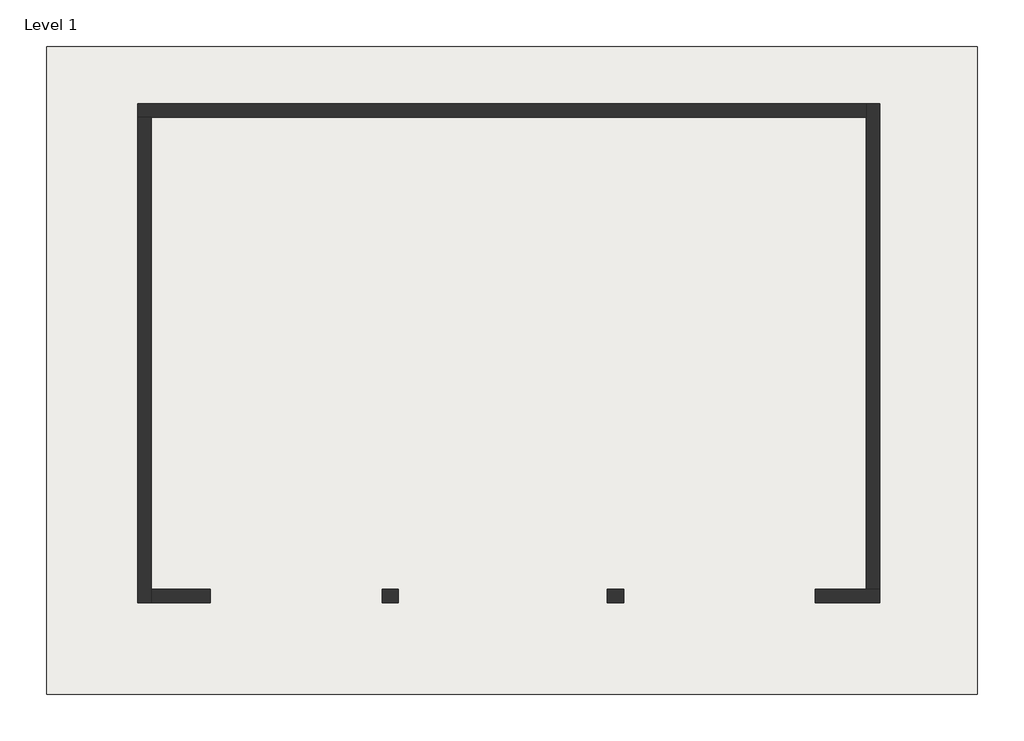
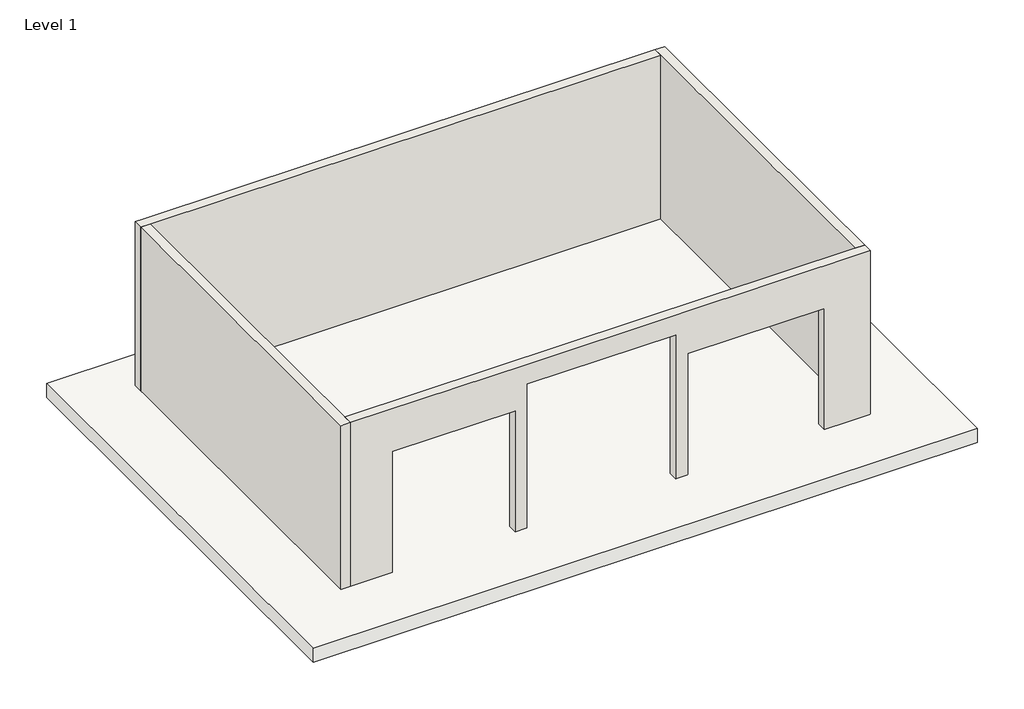
# One storey: 4 walls, 1 slab.
"""IFC4 building model written with IfcOpenShell, lengths in millimetres."""

from ifc_helpers import new_model, si_unit, frame, origin, place, context, project, spatial, polyline, outline, extrude, faceted_brep, element, save

model = new_model("IFC4")

# Units and contexts
model_context = context("Model", 3, world=origin())
ifc_project = project(units=[si_unit("LENGTHUNIT", "METRE", prefix="MILLI")], contexts=[model_context])

# Site, building, storey
site = spatial("IfcSite", under=ifc_project)
building = spatial("IfcBuilding", under=site)
storey = spatial("IfcBuildingStorey", under=building, Name="Level 1", Elevation=0.0)

# Slab
placement = place(None, origin())
element("IfcSlab", 1, ObjectType="Generic - 12\"", at=placement, inside=storey, context=model_context, shape_type="SweptSolid", body=[
    extrude(outline(polyline([(1630.1130714, 10293.742324), (1630.1130714, 540.142324), (-12390.6869286, 540.142324), (-12390.6869286, 10293.742324), (1630.1130714, 10293.742324)])), frame((0.0, 0.0, -304.8), z_axis=(0.0, 0.0, 1.0), x_axis=(1.0, 0.0, 0.0)), (0.0, 0.0, 1.0), 304.8),
])

# Walls
element("IfcWall", 2, ObjectType="Generic - 8\"", at=placement, inside=storey, context=model_context, shape_type="Brep", body=[
    faceted_brep([(-11016.1183714, 9229.4236997, 0.0), (-10812.9183714, 9229.4236997, 0.0), (-43.3183714, 9229.4236997, 0.0), (-43.3183714, 9229.4236997, 3657.6), (-10812.9183714, 9229.4236997, 3657.6), (-11016.1183714, 9229.4236997, 3657.6), (-11016.1183714, 9432.6236997, 0.0), (-11016.1183714, 9432.6236997, 3657.6), (-10812.9183714, 9432.6236997, 3657.6), (-43.3183714, 9432.6236997, 3657.6), (-43.3183714, 9432.6236997, 0.0)], [[[0, 1, 2, 3, 4, 5]], [[6, 7, 8, 9, 10]], [[2, 1, 0, 6, 10]], [[0, 5, 7, 6]], [[2, 10, 9, 3]], [[7, 5, 4, 3, 9, 8]]]),
])
element("IfcWall", 3, ObjectType="Generic - 8\"", at=placement, inside=storey, context=model_context, shape_type="Brep", body=[
    faceted_brep([(-10812.9183714, 1914.2236997, 0.0), (-10812.9183714, 2117.4236997, 0.0), (-10812.9183714, 9229.4236997, 0.0), (-10812.9183714, 9229.4236997, 3657.6), (-10812.9183714, 3641.4236997, 3657.6), (-10812.9183714, 2117.4236997, 3657.6), (-10812.9183714, 1914.2236997, 3657.6), (-11016.1183714, 1914.2236997, 0.0), (-11016.1183714, 1914.2236997, 3657.6), (-11016.1183714, 3641.4236997, 3657.6), (-11016.1183714, 9229.4236997, 3657.6), (-11016.1183714, 9229.4236997, 0.0)], [[[0, 1, 2, 3, 4, 5, 6]], [[7, 8, 9, 10, 11]], [[2, 1, 0, 7, 11]], [[0, 6, 8, 7]], [[6, 5, 4, 3, 10, 9, 8]], [[2, 11, 10, 3]]]),
])
element("IfcWall", 4, ObjectType="Generic - 8\"", at=placement, inside=storey, context=model_context, shape_type="Brep", body=[
    faceted_brep([(159.8816286, 2117.4236997, 0.0), (-43.3183714, 2117.4236997, 0.0), (-810.5509081, 2117.4236997, 0.0), (-810.5509081, 2117.4236997, 2705.2884148), (-3696.009562, 2117.4236997, 2705.2884148), (-3696.009562, 2117.4236997, 0.0), (-3948.2087885, 2117.4236997, 0.0), (-3948.2087885, 2117.4236997, 3216.7013864), (-7091.896639, 2117.4236997, 3216.7013864), (-7091.896639, 2117.4236997, 0.0), (-7336.9262238, 2117.4236997, 0.0), (-7336.9262238, 2117.4236997, 2705.2884148), (-9928.4032219, 2117.4236997, 2705.2884148), (-9928.4032219, 2117.4236997, 0.0), (-10812.9183714, 2117.4236997, 0.0), (-10812.9183714, 2117.4236997, 3657.6), (-43.3183714, 2117.4236997, 3657.6), (159.8816286, 2117.4236997, 3657.6), (159.8816286, 1914.2236997, 0.0), (159.8816286, 1914.2236997, 3657.6), (-3948.2087885, 1914.2236997, 3657.6), (-7091.896639, 1914.2236997, 3657.6), (-10812.9183714, 1914.2236997, 3657.6), (-10812.9183714, 1914.2236997, 0.0), (-9928.4032219, 1914.2236997, 0.0), (-9928.4032219, 1914.2236997, 2705.2884148), (-7336.9262238, 1914.2236997, 2705.2884148), (-7336.9262238, 1914.2236997, 0.0), (-7091.896639, 1914.2236997, 0.0), (-7091.896639, 1914.2236997, 3216.7013864), (-3948.2087885, 1914.2236997, 3216.7013864), (-3948.2087885, 1914.2236997, 0.0), (-3696.009562, 1914.2236997, 0.0), (-3696.009562, 1914.2236997, 2705.2884148), (-810.5509081, 1914.2236997, 2705.2884148), (-810.5509081, 1914.2236997, 0.0)], [[[0, 1, 2, 3, 4, 5, 6, 7, 8, 9, 10, 11, 12, 13, 14, 15, 16, 17]], [[18, 19, 20, 21, 22, 23, 24, 25, 26, 27, 28, 29, 30, 31, 32, 33, 34, 35]], [[0, 17, 19, 18]], [[15, 14, 23, 22]], [[17, 16, 15, 22, 21, 20, 19]], [[2, 1, 0, 18, 35]], [[3, 2, 35, 34]], [[4, 3, 34, 33]], [[5, 4, 33, 32]], [[11, 10, 27, 26]], [[12, 11, 26, 25]], [[13, 12, 25, 24]], [[14, 13, 24, 23]], [[6, 5, 32, 31]], [[7, 6, 31, 30]], [[8, 7, 30, 29]], [[9, 8, 29, 28]], [[10, 9, 28, 27]]]),
])
element("IfcWall", 5, ObjectType="Generic - 8\"", at=placement, inside=storey, context=model_context, shape_type="Brep", body=[
    faceted_brep([(-43.3183714, 9432.6236997, 0.0), (-43.3183714, 9229.4236997, 0.0), (-43.3183714, 2117.4236997, 0.0), (-43.3183714, 2117.4236997, 3657.6), (-43.3183714, 3489.0236997, 3657.6), (-43.3183714, 9229.4236997, 3657.6), (-43.3183714, 9432.6236997, 3657.6), (159.8816286, 9432.6236997, 0.0), (159.8816286, 9432.6236997, 3657.6), (159.8816286, 9229.4236997, 3657.6), (159.8816286, 3489.0236997, 3657.6), (159.8816286, 2117.4236997, 3657.6), (159.8816286, 2117.4236997, 0.0)], [[[0, 1, 2, 3, 4, 5, 6]], [[7, 8, 9, 10, 11, 12]], [[2, 1, 0, 7, 12]], [[3, 2, 12, 11]], [[0, 6, 8, 7]], [[8, 6, 5, 4, 3, 11, 10, 9]]]),
])

save(model, "model.ifc")

# Revit data of these elements
# Type "Generic - 12\""
#   Assembly Code = "B1010"
#   Function = 0
#   Layers, outside or top first: 1' - 0" no material (function 1)
# Type "Generic - 8\""
#   Assembly Code = "B2010"
#   Layers, outside or top first: 0' - 8" no material (function 1)
# Element 1 (IfcSlab, "Generic - 12\"")
#   Height Offset From Level = 0' - 0"
#   Phase Created = New Construction
#   Materials on its faces: "Default Floor"
# Elements 2, 3, 4, 5 (IfcWall, "Generic - 8\"")
#   Top Offset = 0' - 0"
#   Base Offset = 0' - 0"
#   Unconnected Height = 20' - 0"
#   wall height = 20' - 0"
#   Phase Created = New Construction
#   Base Constraint = Level 1
#   Materials on its faces: "Default Wall"
# Materials
#   "Default Floor": colour RGB 128 128 128, transparency 0
#   "Default Wall": colour RGB 128 128 128, transparency 0
